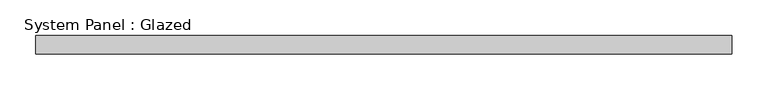
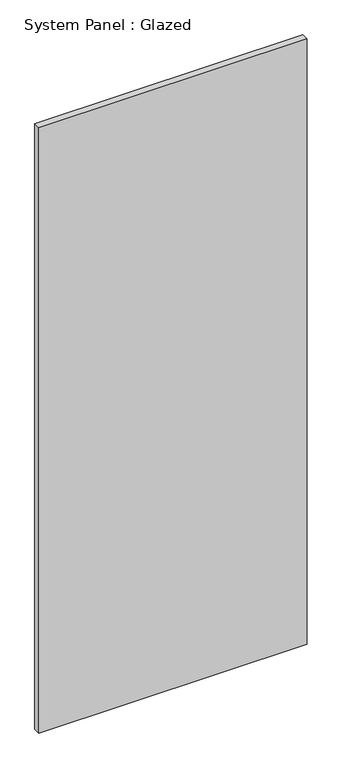
"""IFC4 building model written with IfcOpenShell, lengths in millimetres: plate geometry, System Panel : Glazed."""

from ifc_helpers import new_model, si_unit, origin, origin_with_axes, place, context, project, spatial, polyline, outline, extrude, source, transform, mapped, element, save


def system_panel_glazed_d119973b(model_context):
    return source(origin(), model_context, "Body", "SweptSolid", [
        extrude(outline(polyline([(485.775, 19.05), (-485.775, 19.05), (-485.775, 44.45), (485.775, 44.45), (485.775, 19.05)])), origin_with_axes(), (0.0, 0.0, 1.0), 2318.7520936),
    ])


if __name__ == "__main__":
    model = new_model("IFC4")
    model_context = context("Model", 3, world=origin())
    ifc_project = project(units=[si_unit("LENGTHUNIT", "METRE", prefix="MILLI")], contexts=[model_context])
    site = spatial("IfcSite", under=ifc_project)
    building = spatial("IfcBuilding", under=site)
    placement = place(None, origin())
    system_panel_glazed_shape = system_panel_glazed_d119973b(model_context)
    element("IfcPlate", 1, ObjectType="System Panel : Glazed", at=placement, inside=building, context=model_context, shape_type="MappedRepresentation", body=[
        mapped(system_panel_glazed_shape, transform((0.0, 0.0, 0.0), x_axis=(1.0, 0.0, 0.0), y_axis=(0.0, 1.0, 0.0), z_axis=(0.0, 0.0, 1.0))),
    ])
    save(model, "model.ifc")

# Revit data of these elements
# Type "System Panel : Glazed"
#   Construction Type Id = "GSP4R"
#   Analytic Construction = "1/8 in Pilkington single glazing"
#   Visual Light Transmittance = 0.9
#   Solar Heat Gain Coefficient = 0.86
#   Heat Transfer Coefficient (U) = 1.18115 BTU/(h·ft²·°F)
#   Define Thermal Properties by = 1
# Element 1 (IfcPlate, "System Panel : Glazed")
#   Materials on its faces: "Glass"
# Materials
#   "Glass": class "Glass", colour RGB 0 128 192, transparency 0.75, Description = "Soda Lime Glass", Cost = 0
